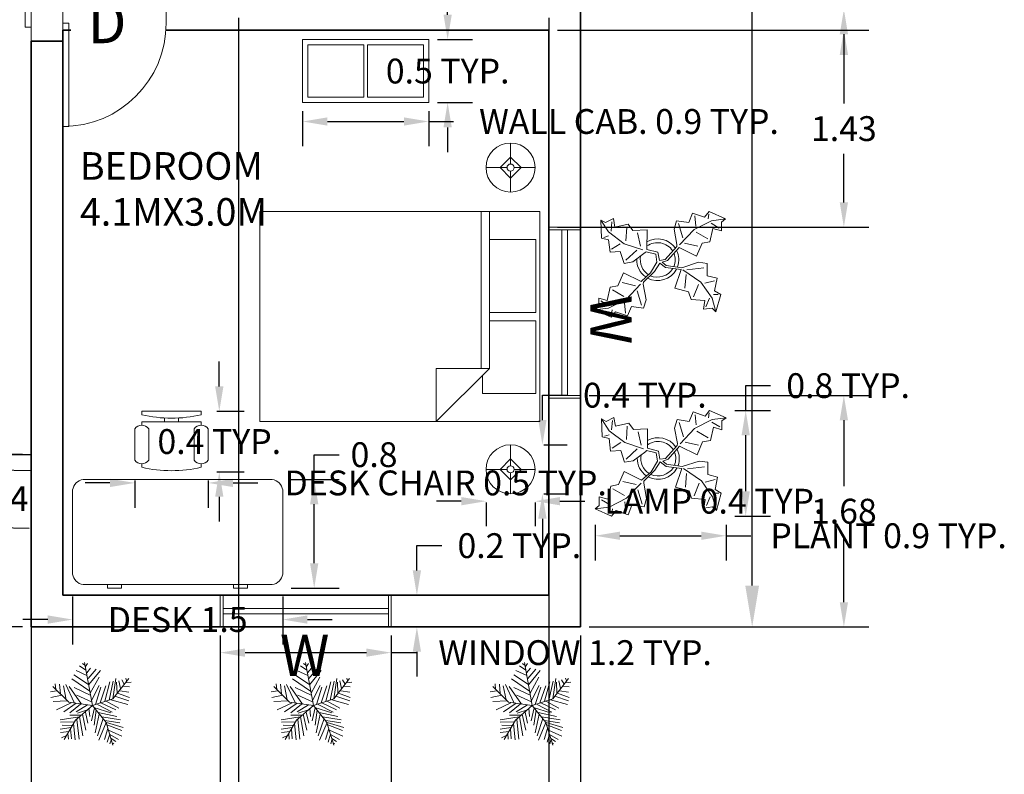
# Model space of a CAD drawing. Units: metres. Extents: x 40.9 to 56.1, y -1.4 to 24.2.
# Tile 4 of 7: x 48.4 to 55.6, y 7.6 to 13.1. Entities that reach past the tile are written whole.
import ezdxf

# ---------------------------------------------------------------- set-up
doc = ezdxf.new("R2010")
doc.units = ezdxf.units.M
doc.header["$MEASUREMENT"] = 0
for name, color, linetype, lineweight in [('A-ANNO-DIMS', 2, 'Continuous', 18), ('A-ANNO-TEXT', 7, 'Continuous', 18), ('A-AREA-IDEN', 7, 'Continuous', 18), ('A-DOOR', 3, 'Continuous', 18), ('A-FLOR', 7, 'Continuous', 25), ('A-FLOR-CASE', 9, 'Continuous', 18), ('A-FURN', 8, 'Continuous', 18), ('A-GLAZ', 4, 'Continuous', 18), ('A-WALL', 7, 'Continuous', 35), ('L-PLNT', 94, 'Continuous', 13)]:
    doc.layers.add(name, color=color, linetype=linetype, lineweight=lineweight)
doc.styles.get("Standard").update_dxf_attribs({"font": 'arial.ttf'})
doc.dimstyles.get("Standard").update_dxf_attribs({"dimtxt": 0.18, "dimasz": 0.18, "dimexe": 0.18, "dimexo": 0.0625, "dimgap": 0.09, "dimtad": 0, "dimtih": 1, "dimtoh": 1, "dimdec": 1, "dimzin": 0, "dimdsep": 46, "dimtxsty": 'Standard', "dimcen": 0.09, "dimadec": 0, "dimazin": 0, "dimtfac": 1, "dimtdec": 1, "dimtofl": 0, "dimtmove": 0, "dimatfit": 3, "dimfxl": 1, "dimtolj": 1, "dimtzin": 0, "dimarcsym": 0})

# ---------------------------------------------------------------- blocks, each defined once
blk = doc.blocks.new('*U3')
for p, q in [((-750, 0), (-750, -100)), ((0, 0), (0, -100))]:
    blk.add_line(p, q)
blk.add_lwpolyline([(0, 0), (0, 750), (-43.75, 750), (-43.75, 0)], close=True)
blk.add_arc((0, 0), 750, 90, 180)
blk = doc.blocks.new('*U4')
for p, q in [((0, 0), (0, 100)), ((750, 0), (750, 100))]:
    blk.add_line(p, q)
blk.add_lwpolyline([(0, 0), (0, -750), (43.75, -750), (43.75, 0)], close=True)
blk.add_arc((0, 0), 750, 270, 0)
blk = doc.blocks.new('Bed - Queen')
for p, q in [((0, -80.00003), (0, 0)), ((0, 0), (59.99999, 0)), ((59.99999, 0), (59.99999, -80.00003)), ((7.99999, -1.2), (28.79998, -1.2)), ((7.99999, -14.4), (7.99999, -1.2)), ((28.79998, -1.2), (28.79998, -14.4)), ((31.19999, -1.2), (51.99999, -1.2)), ((31.19999, -14.4), (31.19999, -1.2)), ((51.99999, -1.2), (51.99999, -16.4)), ((0, -14.4), (44.8, -14.4)), ((44.8, -16.8), (0, -16.8)), ((59.99999, -29.6), (44.8, -14.4)), ((44.8, -14.4), (44.8, -29.6)), ((51.99999, -16.4), (46.79936, -16.4)), ((44.8, -29.6), (59.99999, -29.6)), ((59.99999, -80.00003), (0, -80.00003))]:
    blk.add_line(p, q)
blk = doc.blocks.new('Lamp - Table')
for p, q in [((0, 7), (0, 1)), ((0, 3), (-3, 0)), ((3, 0), (0, 3)), ((-1, 0), (-7, 0)), ((-3, 0), (0, -3)), ((0, -3), (3, 0)), ((1, 0), (7, 0)), ((0, -1), (0, -7))]:
    blk.add_line(p, q)
for radius in [7, 1]:
    blk.add_circle((0, 0), radius)
blk = doc.blocks.new('Chair - Desk')
for p, q in [((-8.5, 0), (-8.5, -1)), ((-8.5, 0), (8.5, 0)), ((8.5, 0), (8.5, -1)), ((-2, -3), (-2, -1.9355)), ((2, -1.9576), (2, -3)), ((-10.5, -5), (-10.5, -14)), ((-8.5, -3), (-8.5, -4)), ((-8.5, -3), (8.5, -3)), ((-6.5, -14), (-6.5, -5)), ((6.5, -5), (6.5, -14)), ((8.5, -3), (8.5, -4)), ((10.5, -14), (10.5, -5)), ((-8.5, -15), (-8.5, -16)), ((8.5, -15), (8.5, -16))]:
    blk.add_line(p, q)
for centre, radius, start, end in [((0, 34.625), 36.625, 256.5803, 283.4197), ((-8.5, -6.5), 2.5, 36.8699, 143.1301), ((8.5, -6.5), 2.5, 36.8699, 143.1301), ((-8.5, -12.5), 2.5, 216.8699, 323.1301), ((8.5, -12.5), 2.5, 216.8699, 323.1301), ((0, 19.625), 36.625, 256.5803, 283.4197)]:
    blk.add_arc(centre, radius, start, end)
blk = doc.blocks.new('Desk - 30 x 60 in.')
for p, q in [((-26.999995, 0), (26.999995, 0)), ((-29.999995, -27), (-29.999995, -3)), ((29.999995, -3), (29.999995, -27)), ((26.999995, -30), (-26.999995, -30)), ((-20.000005, -30), (-20.000005, -31)), ((-16.000005, -31), (-16.000005, -30)), ((15.999995, -31), (15.999995, -30)), ((19.999995, -30), (19.999995, -31)), ((-20.000005, -31), (-16.000005, -31)), ((19.999995, -31), (15.999995, -31))]:
    blk.add_line(p, q)
for centre, start, end in [((-26.499995, -3.5), 98.1301, 171.8699), ((26.499995, -3.5), 8.130102, 81.8699), ((-26.499995, -26.5), 188.1301, 261.8699), ((26.499995, -26.5), 278.1301, 351.8699)]:
    blk.add_arc(centre, 3.535534, start, end)
blk = doc.blocks.new('Wall Cabinet - 18 x 36 in front')
for p, q in [((17.5, -1.5), (17.5, -16.5)), ((18.5, -16.5), (18.5, -1.5))]:
    blk.add_line(p, q)
blk.add_lwpolyline([(0, -18), (0, 0), (36, 0), (36, -18)], close=True)
for points in [[(17.5, -16.5), (1.5, -16.5), (1.5, -1.5), (17.5, -1.5)], [(18.5, -1.5), (34.5, -1.5), (34.5, -16.5), (18.5, -16.5)]]:
    blk.add_lwpolyline(points)
blk = doc.blocks.new('*U26')
for p, q in [((-221.9198, 1197.3052), (-433.5526, 1338.8594)), ((-258.7244, 1362.456), (-332.3336, 1421.4348)), ((0, 0), (-266.7, 1447.8)), ((-231.1146, 1315.2628), (-166.7002, 1421.4348)), ((-129.8956, 713.6638), (-626.7704, 1032.1544)), ((-185.1152, 1008.5578), (-553.1612, 1185.4942)), ((-194.31, 1102.9442), (-65.4812, 1256.284)), ((-148.3106, 914.1968), (118.5418, 1220.9018)), ((-129.8956, 701.8528), (265.7602, 1185.4942)), ((-1234.059, 536.7274), (-1252.4486, 737.2604)), ((-1105.2302, 725.4494), (-1077.6458, 395.1732)), ((-976.4268, 666.4706), (-884.4026, 194.6402)), ((-902.8176, 713.6638), (-617.5756, 100.2538)), ((-93.091, 489.5342), (-700.3796, 902.3858)), ((-74.7014, 418.7444), (219.7608, 961.39)), ((-28.6766, 171.0436), (228.9556, 678.2816)), ((256.5654, 88.4682), (449.7832, 666.4706)), ((412.9786, 147.447), (587.8068, 796.2392)), ((560.197, 182.8292), (698.2206, 819.8358)), ((685.8, 228.6), (1219.2, 914.4)), ((689.0258, 230.0224), (790.2448, 914.1968)), ((808.6344, 784.4282), (827.0494, 418.7444)), ((891.4384, 831.6214), (946.658, 572.1096)), ((983.4626, 867.0036), (1066.2666, 725.4494)), ((1112.2914, 760.8316), (1296.3144, 784.4282)), ((1121.4862, 925.9824), (1149.0706, 831.6214)), ((-1206.4492, 501.3198), (-1418.082, 465.9376)), ((-1031.621, 347.98), (-1399.667, 277.1902)), ((-800.1, 114.3), (-1333.5, 647.7)), ((-369.1382, 53.086), (-783.1836, 642.874)), ((-617.5756, 607.4918), (-74.7014, 347.98)), ((-525.5514, 347.98), (-28.6766, 123.8504)), ((100.1268, 41.275), (284.1498, 619.2774)), ((845.439, 418.7444), (1241.0948, 277.1902)), ((919.0482, 501.3198), (1222.6798, 454.152)), ((1029.462, 654.685), (1241.0948, 631.0884)), ((-847.598, 159.2326), (-1326.0578, 135.636)), ((-718.7946, 88.4682), (-1215.644, -147.447)), ((-543.9664, 76.6572), (-967.2066, -206.4512)), ((0, 0), (-800.1, 114.3)), ((-405.9428, 53.086), (-764.794, -241.8334)), ((0, 0), (-571.5, -495.3)), ((-166.7002, 29.4894), (-543.9664, -206.4512)), ((0, 0), (685.8, 228.6)), ((0, 0), (457.2, -571.5)), ((164.5412, 41.275), (661.416, -218.2368)), ((284.1498, 88.4682), (781.0246, -147.447)), ((458.978, 147.447), (891.4384, -88.4682)), ((615.4166, 194.6402), (1185.8752, 41.275)), ((753.4148, 312.5978), (1222.6798, 159.2326)), ((-387.5278, -324.4088), (-764.794, -324.4088)), ((-166.7002, -147.447), (-507.1618, -253.619)), ((-341.5284, -289.0012), (-221.9198, -831.6214)), ((-240.3094, -218.2368), (-157.5054, -595.7062)), ((-120.7008, -88.4682), (-93.091, -371.5766)), ((63.3222, -76.6826), (-37.8714, -513.1308)), ((44.9326, -64.897), (615.4166, -241.8334)), ((127.7366, -159.258), (54.1274, -654.685)), ((228.9556, -289.0012), (90.932, -914.1968)), ((192.151, -230.0224), (817.8292, -371.5766)), ((-442.7474, -383.3876), (-1086.8406, -477.7486)), ((-617.5756, -548.5384), (-1077.6458, -560.324)), ((-681.9646, -666.496), (-1022.4262, -654.685)), ((-571.5, -495.3), (-952.5, -1143)), ((-635.9652, -607.5172), (-580.771, -1150.1374)), ((-525.5514, -465.963), (-451.9422, -1126.5408)), ((-433.5526, -383.3876), (-323.1134, -1020.3688)), ((357.759, -430.5554), (164.5412, -1020.3688)), ((458.978, -572.1096), (210.5406, -1161.923)), ((311.7596, -383.3876), (937.4378, -477.7486)), ((412.9786, -501.3452), (919.0482, -583.9206)), ((457.2, -571.5), (685.8, -1333.5)), ((468.1982, -572.1096), (1029.462, -737.2604)), ((486.5878, -642.8994), (983.4626, -843.4324)), ((-718.7946, -737.2604), (-1086.8406, -796.2392)), ((-783.1836, -867.029), (-1077.6458, -902.4112)), ((-829.2084, -937.7934), (-810.7934, -1126.5408)), ((-737.1842, -784.4536), (-709.5744, -1114.7298)), ((514.1976, -772.6426), (403.7838, -1138.3264)), ((578.612, -961.39), (495.7826, -1232.7128)), ((541.8074, -831.6214), (992.6574, -1032.1544)), ((578.612, -973.1756), (873.0488, -1138.3264)), ((-875.2078, -1008.5832), (-1040.8412, -1079.3476)), ((624.6114, -1161.923), (587.8068, -1291.6916)), ((624.6114, -1102.9442), (781.0246, -1209.1162)), ((679.8056, -1268.095), (716.6102, -1291.6916))]:
    blk.add_line(p, q)
blk = doc.blocks.new('Plant - Rubber or Philodendron')
for p, q in [((-16.2005, 11.4774), (-13.9899, 8.1064)), ((-16.2005, 11.4774), (-14.8639, 10.7964)), ((-16.0159, 6.3329), (-16.2005, 11.4774)), ((-14.8639, 10.7964), (-12.6195, 11.8975)), ((-12.6195, 11.8975), (-12.1909, 9.4345)), ((4.6914, 8.8812), (5.3859, 11.2828)), ((5.3859, 11.2828), (8.8871, 10.7908)), ((8.8871, 10.7908), (9.9809, 13.4933)), ((9.9809, 13.4933), (13.3837, 12.301)), ((15.3859, 11.3055), (10.3916, 8.7942)), ((10.5828, 12.6946), (10.8893, 9.7953)), ((13.3837, 12.301), (14.68, 13.9039)), ((14.5816, 13.2037), (14.3848, 11.8033)), ((14.68, 13.9039), (19.3848, 11.8146)), ((19.3848, 11.8146), (15.3859, 11.3055)), ((19.3848, 11.8146), (18.1868, 10.9119)), ((-13.3174, 8.325), (-13.0735, 11.0065)), ((-12.1909, 9.4345), (-8.3829, 10.3)), ((-8.8369, 9.409), (-9.0894, 5.6095)), ((-8.3829, 10.3), (-7.0549, 8.501)), ((-7.0549, 8.501), (-3.0284, 8.6941)), ((-3.0284, 8.6941), (-3.0709, 3.1041)), ((4.6914, 8.8812), (5.5014, 4.4831)), ((5.9878, 10.4842), (7.1971, 6.3869)), ((10.3916, 8.7942), (6.2847, 4.4028)), ((15.7909, 9.1065), (14.8995, 5.3044)), ((15.2875, 10.6053), (17.5907, 9.2105)), ((18.1925, 8.4119), (15.7909, 9.1065)), ((18.1868, 10.9119), (18.1925, 8.4119)), ((-14.0069, 5.8704), (-16.0159, 6.3329)), ((-15.3434, 6.5514), (-13.9984, 6.9884)), ((-13.5868, 2.2894), (-14.0069, 5.8704)), ((-13.9899, 8.1064), (-9.5434, 4.7185)), ((-4.8529, 4.012), (-5.7184, 7.82)), ((14.2977, 6.1031), (10.9934, 7.9956)), ((-13.1329, 3.1804), (-10.6614, 4.727)), ((-9.5434, 4.7185), (-4.1917, 2.9888)), ((-9.1318, 0.0195), (-5.9793, 2.9025)), ((-3.0709, 3.1041), (0.0797, 2.3163)), ((2.1141, 0.2298), (5.4346, 3.9146)), ((6.1032, 3.6844), (2.8262, -0.031)), ((5.4346, 3.9146), (5.5014, 4.4831)), ((11.1089, 1.1958), (6.1032, 3.6844)), ((7.7005, 4.8881), (11.5025, 3.9967)), ((12.7005, 4.8994), (11.1089, 1.1958)), ((14.8995, 5.3044), (12.7005, 4.8994)), ((-10.6784, 2.491), (-13.5868, 2.2894)), ((-9.5858, -0.8715), (-10.6784, 2.491)), ((-7.1228, -0.443), (-3.5248, 2.2131)), ((-3.5248, 2.2131), (-3.3011, 2.4355)), ((-3.3011, 2.4355), (-0.5306, 1.7947)), ((-0.5306, 1.7947), (-0.2255, -0.5527)), ((-0.5306, 1.7947), (-0.5306, 1.7947)), ((0.0797, 2.3163), (0.4866, -0.031)), ((0.4866, -0.031), (2.1141, 0.2298)), ((-7.1228, -0.443), (-9.5858, -0.8715)), ((-2.019, -3.6148), (-0.2255, -0.5527)), ((-0.9375, -3.1608), (0.5883, -0.8135)), ((0.5883, -0.8135), (2.2447, -2.0916)), ((2.8262, -0.031), (1.3003, -0.5527)), ((1.3003, -0.5527), (2.4193, -1.4655)), ((2.2447, -2.0916), (6.7108, -2.6626)), ((2.4193, -1.4655), (6.895, -2.1175)), ((4.943, -7.9659), (6.7108, -2.6626)), ((11.6605, -0.5413), (6.895, -2.1175)), ((12.3677, -6.1981), (7.219, -2.6772)), ((8.3544, -2.7453), (13.1973, -2.1704)), ((11.6605, -0.5413), (14.1354, -0.8948)), ((14.1354, -0.8948), (14.1354, -4.4304)), ((-11.3237, -7.2629), (-9.7321, -3.5593)), ((-9.7321, -3.5593), (-4.7264, -6.0479)), ((-2.019, -3.6148), (-4.7264, -6.0479)), ((-4.0579, -6.2781), (-0.9375, -3.1608)), ((8.125, -4.0768), (7.7715, -7.9659)), ((14.1354, -4.4304), (16.9638, -5.1375)), ((16.9638, -5.1375), (16.2567, -8.673)), ((-14.4141, -11.4699), (-13.5228, -7.6679)), ((-13.5228, -7.6679), (-11.3237, -7.2629)), ((-6.3237, -7.2516), (-10.1257, -6.3602)), ((-9.0148, -11.1577), (-4.9047, -6.8122)), ((-4.1246, -6.8466), (-4.0579, -6.2781)), ((-3.3146, -11.2447), (-4.1246, -6.8466)), ((8.8321, -9.0266), (4.943, -7.9659)), ((10.2463, -10.4408), (11.6605, -6.9053)), ((15.5496, -10.7943), (12.3677, -6.1981)), ((16.2567, -5.8446), (13.4283, -6.5517)), ((-16.8157, -10.7754), (-14.4141, -11.4699)), ((-16.8101, -13.2754), (-16.8157, -10.7754)), ((-14.0091, -13.669), (-9.0148, -11.1577)), ((-12.921, -8.4665), (-9.6166, -10.359)), ((-4.611, -12.8477), (-5.8203, -8.7504)), ((-3.3146, -11.2447), (-4.0092, -13.6463)), ((9.5392, -11.1479), (8.8321, -9.0266)), ((13.4283, -11.5015), (9.5392, -11.1479)), ((14.8425, -10.7943), (13.7819, -13.2692)), ((16.6103, -14.6834), (15.5496, -10.7943)), ((17.3174, -9.7337), (15.9032, -9.7337)), ((16.2567, -8.673), (18.0245, -9.7337)), ((18.0245, -9.7337), (16.6103, -14.6834)), ((-18.008, -14.1781), (-16.8101, -13.2754)), ((-18.008, -14.1781), (-14.0091, -13.669)), ((-13.9107, -12.9688), (-16.2139, -11.574)), ((-9.206, -15.0581), (-9.5126, -12.1588)), ((-7.5103, -13.1543), (-8.6042, -15.8568)), ((-4.0092, -13.6463), (-7.5103, -13.1543)), ((13.0748, -13.9763), (13.4283, -11.5015)), ((15.5496, -13.6228), (13.0748, -13.9763)), ((16.6103, -14.6834), (15.5496, -13.6228)), ((-13.3032, -16.2674), (-18.008, -14.1781)), ((-12.0069, -14.6645), (-13.3032, -16.2674)), ((-13.2048, -15.5672), (-13.008, -14.1668)), ((-8.6042, -15.8568), (-12.0069, -14.6645))]:
    blk.add_line(p, q)
for centre, radius, start, end in [((0, 0), 6.1275, 34.37569, 120.1028), ((-0.0601, -0.2075), 5.2461, 33.82192, 124.9414), ((-0.098, 0.1364), 6.1288, 341.2017, 26.09184), ((0.0308, 0.1664), 6, 178.6147, 235.1169), ((0.0308, 0.1664), 5, 168.1647, 238.6725), ((-0.2664, 0.1682), 5.2775, 338.4094, 20.03007), ((-0.0234, 0.3825), 6.1492, 242.5812, 331.2714), ((-0.1102, 0.4886), 5.2883, 247.3711, 327.472)]:
    blk.add_arc(centre, radius, start, end)
blk = doc.blocks.new('*D46')
at = {"layer": 'A-ANNO-DIMS', "color": 0, "lineweight": -2, "transparency": 16777216}
for p, q in [((52.5777, 22.5873), (53.9408, 22.5873)), ((53.7608, 22.2873), (53.7608, 15.8755)), ((53.7608, 8.9773), (53.7608, 15.389)), ((52.5777, 8.6773), (53.9408, 8.6773))]:
    blk.add_line(p, q, dxfattribs=at)
at = {"layer": 'A-ANNO-DIMS', "color": 0, "transparency": 16777216}
for points in [[(53.7108, 22.2873), (53.8108, 22.2873), (53.7608, 22.5873)], [(53.7108, 8.9773), (53.8108, 8.9773), (53.7608, 8.6773)]]:
    blk.add_solid(points, dxfattribs=at)
at = {"layer": 'Defpoints', "color": 0, "transparency": 16777216}
for p in [(52.5152, 22.5873), (52.5152, 8.6773), (53.7608, 8.6773)]:
    blk.add_point(p, dxfattribs=at)
at = {"layer": 'A-ANNO-DIMS', "color": 0, "transparency": 16777216, "insert": (53.7608, 15.6323), "char_height": 0.3, "attachment_point": 5}
blk.add_mtext('\\A1;13.9', dxfattribs=at)
blk = doc.blocks.new('WIN-1200-PLAN')
for p, q in [((-0.0002, 0.0003), (-0.0002, 0.2303)), ((0.0198, 0.0003), (0.0198, 0.2303)), ((1.2198, 0.0003), (1.2198, 0.2303)), ((1.2398, 0.0003), (1.2398, 0.2303)), ((0.0198, 0.1353), (1.2198, 0.1353)), ((0.0198, 0.0953), (1.2198, 0.0953))]:
    blk.add_line(p, q)
blk = doc.blocks.new('*D73')
at = {"layer": 'A-ANNO-DIMS', "color": 0, "lineweight": -2, "transparency": 16777216}
for p, q in [((49.9027, 8.6148), (49.9027, 8.3113)), ((51.1427, 8.6148), (51.1427, 8.3113)), ((50.0827, 8.4913), (50.9627, 8.4913)), ((51.1427, 8.4913), (51.3227, 8.4913))]:
    blk.add_line(p, q, dxfattribs=at)
at = {"layer": 'A-ANNO-DIMS', "color": 0, "transparency": 16777216}
for points in [[(50.0827, 8.5213), (50.0827, 8.4613), (49.9027, 8.4913)], [(50.9627, 8.5213), (50.9627, 8.4613), (51.1427, 8.4913)]]:
    blk.add_solid(points, dxfattribs=at)
at = {"layer": 'Defpoints', "color": 0, "transparency": 16777216}
for p in [(49.9027, 8.6773), (51.1427, 8.6773), (51.1427, 8.4913)]:
    blk.add_point(p, dxfattribs=at)
at = {"layer": 'A-ANNO-DIMS', "color": 0, "transparency": 16777216, "insert": (52.476, 8.4913), "char_height": 0.18, "attachment_point": 5}
blk.add_mtext('\\A1;WINDOW 1.2 TYP.', dxfattribs=at)
blk = doc.blocks.new('*D74')
at = {"layer": 'A-ANNO-DIMS', "color": 0, "lineweight": -2, "transparency": 16777216}
for p, q in [((51.3287, 9.0873), (51.3287, 9.2673)), ((51.3287, 9.2673), (51.5087, 9.2673)), ((51.2052, 8.9073), (51.5087, 8.9073)), ((51.2052, 8.6773), (51.5087, 8.6773)), ((51.3287, 8.4973), (51.3287, 8.3173))]:
    blk.add_line(p, q, dxfattribs=at)
at = {"layer": 'A-ANNO-DIMS', "color": 0, "transparency": 16777216}
for points in [[(51.2987, 9.0873), (51.3587, 9.0873), (51.3287, 8.9073)], [(51.2987, 8.4973), (51.3587, 8.4973), (51.3287, 8.6773)]]:
    blk.add_solid(points, dxfattribs=at)
at = {"layer": 'Defpoints', "color": 0, "transparency": 16777216}
for p in [(51.1427, 8.9073), (51.3287, 8.9073), (51.1427, 8.6773)]:
    blk.add_point(p, dxfattribs=at)
at = {"layer": 'A-ANNO-DIMS', "color": 0, "transparency": 16777216, "insert": (52.0717, 9.2673), "char_height": 0.18, "attachment_point": 5}
blk.add_mtext('\\A1;0.2 TYP.', dxfattribs=at)
blk = doc.blocks.new('*D81')
at = {"layer": 'A-ANNO-DIMS', "color": 0, "lineweight": -2, "transparency": 16777216}
for p, q in [((51.6504, 9.5897), (51.4704, 9.5897)), ((51.8304, 9.5805), (51.8304, 9.4097)), ((52.186, 9.5805), (52.186, 9.4097)), ((52.366, 9.5897), (52.546, 9.5897))]:
    blk.add_line(p, q, dxfattribs=at)
at = {"layer": 'A-ANNO-DIMS', "color": 0, "transparency": 16777216}
for points in [[(51.6504, 9.6197), (51.6504, 9.5597), (51.8304, 9.5897)], [(52.366, 9.6197), (52.366, 9.5597), (52.186, 9.5897)]]:
    blk.add_solid(points, dxfattribs=at)
at = {"layer": 'Defpoints', "color": 0, "transparency": 16777216}
for p in [(51.8304, 9.643), (52.186, 9.643), (52.186, 9.5897)]:
    blk.add_point(p, dxfattribs=at)
at = {"layer": 'A-ANNO-DIMS', "color": 0, "transparency": 16777216, "insert": (53.4823, 9.5897), "char_height": 0.18, "attachment_point": 5}
blk.add_mtext('\\A1;LAMP 0.4 TYP.', dxfattribs=at)
blk = doc.blocks.new('*D82')
at = {"layer": 'A-ANNO-DIMS', "color": 0, "lineweight": -2, "transparency": 16777216}
for p, q in [((52.2393, 10.1786), (52.2393, 10.3586)), ((52.2393, 10.3586), (52.4193, 10.3586)), ((52.2485, 9.9986), (52.4193, 9.9986)), ((52.2485, 9.643), (52.4193, 9.643)), ((52.2393, 9.463), (52.2393, 9.283))]:
    blk.add_line(p, q, dxfattribs=at)
at = {"layer": 'A-ANNO-DIMS', "color": 0, "transparency": 16777216}
for points in [[(52.2093, 10.1786), (52.2693, 10.1786), (52.2393, 9.9986)], [(52.2093, 9.463), (52.2693, 9.463), (52.2393, 9.643)]]:
    blk.add_solid(points, dxfattribs=at)
at = {"layer": 'Defpoints', "color": 0, "transparency": 16777216}
for p in [(52.186, 9.9986), (52.2393, 9.9986), (52.186, 9.643)]:
    blk.add_point(p, dxfattribs=at)
at = {"layer": 'A-ANNO-DIMS', "color": 0, "transparency": 16777216, "insert": (52.9824, 10.3586), "char_height": 0.18, "attachment_point": 5}
blk.add_mtext('\\A1;0.4 TYP.', dxfattribs=at)
blk = doc.blocks.new('*D83')
at = {"layer": 'A-ANNO-DIMS', "color": 0, "lineweight": -2, "transparency": 16777216}
for p, q in [((49.1021, 9.7223), (48.9221, 9.7223)), ((49.2821, 9.7398), (49.2821, 9.5423)), ((49.8155, 9.7398), (49.8155, 9.5423)), ((49.9955, 9.7223), (50.1755, 9.7223))]:
    blk.add_line(p, q, dxfattribs=at)
at = {"layer": 'A-ANNO-DIMS', "color": 0, "transparency": 16777216}
for points in [[(49.1021, 9.7523), (49.1021, 9.6923), (49.2821, 9.7223)], [(49.9955, 9.7523), (49.9955, 9.6923), (49.8155, 9.7223)]]:
    blk.add_solid(points, dxfattribs=at)
at = {"layer": 'Defpoints', "color": 0, "transparency": 16777216}
for p in [(49.2821, 9.8023), (49.8155, 9.8023), (49.8155, 9.7223)]:
    blk.add_point(p, dxfattribs=at)
at = {"layer": 'A-ANNO-DIMS', "color": 0, "transparency": 16777216, "insert": (51.5375, 9.7223), "char_height": 0.18, "attachment_point": 5}
blk.add_mtext('\\A1;DESK CHAIR 0.5 TYP.', dxfattribs=at)
blk = doc.blocks.new('*D84')
at = {"layer": 'A-ANNO-DIMS', "color": 0, "lineweight": -2, "transparency": 16777216}
for p, q in [((49.8955, 10.4226), (49.8955, 10.6026)), ((49.878, 10.2426), (50.0755, 10.2426)), ((49.878, 9.8023), (50.0755, 9.8023)), ((49.8955, 9.6223), (49.8955, 9.4423))]:
    blk.add_line(p, q, dxfattribs=at)
at = {"layer": 'A-ANNO-DIMS', "color": 0, "transparency": 16777216}
for points in [[(49.8655, 10.4226), (49.9255, 10.4226), (49.8955, 10.2426)], [(49.8655, 9.6223), (49.9255, 9.6223), (49.8955, 9.8023)]]:
    blk.add_solid(points, dxfattribs=at)
at = {"layer": 'Defpoints', "color": 0, "transparency": 16777216}
for p in [(49.8155, 10.2426), (49.8955, 10.2426), (49.8155, 9.8023)]:
    blk.add_point(p, dxfattribs=at)
at = {"layer": 'A-ANNO-DIMS', "color": 0, "transparency": 16777216, "insert": (49.8955, 10.0225), "char_height": 0.18, "attachment_point": 5}
blk.add_mtext('\\A1;0.4 TYP.', dxfattribs=at)
blk = doc.blocks.new('*D85')
at = {"layer": 'A-ANNO-DIMS', "color": 0, "lineweight": -2, "transparency": 16777216}
for p, q in [((50.5003, 12.4186), (50.5003, 12.1639)), ((51.4147, 12.4186), (51.4147, 12.1639)), ((50.6803, 12.3439), (51.2347, 12.3439)), ((51.4147, 12.3439), (51.5947, 12.3439))]:
    blk.add_line(p, q, dxfattribs=at)
at = {"layer": 'A-ANNO-DIMS', "color": 0, "transparency": 16777216}
for points in [[(50.6803, 12.3739), (50.6803, 12.3139), (50.5003, 12.3439)], [(51.2347, 12.3739), (51.2347, 12.3139), (51.4147, 12.3439)]]:
    blk.add_solid(points, dxfattribs=at)
at = {"layer": 'Defpoints', "color": 0, "transparency": 16777216}
for p in [(50.5003, 12.4811), (51.4147, 12.4811), (51.4147, 12.3439)]:
    blk.add_point(p, dxfattribs=at)
at = {"layer": 'A-ANNO-DIMS', "color": 0, "transparency": 16777216, "insert": (52.8671, 12.3439), "char_height": 0.18, "attachment_point": 5}
blk.add_mtext('\\A1;WALL CAB. 0.9 TYP.', dxfattribs=at)
blk = doc.blocks.new('*D86')
at = {"layer": 'A-ANNO-DIMS', "color": 0, "lineweight": -2, "transparency": 16777216}
for p, q in [((51.5519, 13.1183), (51.5519, 13.2983)), ((51.4772, 12.9383), (51.7319, 12.9383)), ((51.4772, 12.4811), (51.7319, 12.4811)), ((51.5519, 12.3011), (51.5519, 12.1211))]:
    blk.add_line(p, q, dxfattribs=at)
at = {"layer": 'A-ANNO-DIMS', "color": 0, "transparency": 16777216}
for points in [[(51.5219, 13.1183), (51.5819, 13.1183), (51.5519, 12.9383)], [(51.5219, 12.3011), (51.5819, 12.3011), (51.5519, 12.4811)]]:
    blk.add_solid(points, dxfattribs=at)
at = {"layer": 'Defpoints', "color": 0, "transparency": 16777216}
for p in [(51.4147, 12.9383), (51.5519, 12.9383), (51.4147, 12.4811)]:
    blk.add_point(p, dxfattribs=at)
at = {"layer": 'A-ANNO-DIMS', "color": 0, "transparency": 16777216, "insert": (51.5519, 12.7097), "char_height": 0.18, "attachment_point": 5}
blk.add_mtext('\\A1;0.5 TYP.', dxfattribs=at)
blk = doc.blocks.new('*D89')
at = {"layer": 'A-ANNO-DIMS', "color": 0, "lineweight": -2, "transparency": 16777216}
for p, q in [((52.6216, 9.419), (52.6216, 9.159)), ((53.5713, 9.419), (53.5713, 9.159)), ((52.8016, 9.339), (53.3913, 9.339)), ((53.5713, 9.339), (53.7513, 9.339))]:
    blk.add_line(p, q, dxfattribs=at)
at = {"layer": 'A-ANNO-DIMS', "color": 0, "transparency": 16777216}
for points in [[(52.8016, 9.369), (52.8016, 9.309), (52.6216, 9.339)], [(53.3913, 9.369), (53.3913, 9.309), (53.5713, 9.339)]]:
    blk.add_solid(points, dxfattribs=at)
at = {"layer": 'Defpoints', "color": 0, "transparency": 16777216}
for p in [(52.6216, 9.4815), (53.5713, 9.4815), (53.5713, 9.339)]:
    blk.add_point(p, dxfattribs=at)
at = {"layer": 'A-ANNO-DIMS', "color": 0, "transparency": 16777216, "insert": (54.7501, 9.339), "char_height": 0.18, "attachment_point": 5}
blk.add_mtext('\\A1;PLANT 0.9 TYP.', dxfattribs=at)
blk = doc.blocks.new('*D90')
at = {"layer": 'A-ANNO-DIMS', "color": 0, "lineweight": -2, "transparency": 16777216}
for p, q in [((53.7138, 10.2479), (53.7138, 10.4279)), ((53.7138, 10.4279), (53.8938, 10.4279)), ((53.6338, 10.2479), (53.8938, 10.2479)), ((53.7138, 9.6615), (53.7138, 10.0679)), ((53.6338, 9.4815), (53.8938, 9.4815))]:
    blk.add_line(p, q, dxfattribs=at)
at = {"layer": 'A-ANNO-DIMS', "color": 0, "transparency": 16777216}
for points in [[(53.6838, 10.0679), (53.7438, 10.0679), (53.7138, 10.2479)], [(53.6838, 9.6615), (53.7438, 9.6615), (53.7138, 9.4815)]]:
    blk.add_solid(points, dxfattribs=at)
at = {"layer": 'Defpoints', "color": 0, "transparency": 16777216}
for p in [(53.5713, 10.2479), (53.7138, 10.2479), (53.5713, 9.4815)]:
    blk.add_point(p, dxfattribs=at)
at = {"layer": 'A-ANNO-DIMS', "color": 0, "transparency": 16777216, "insert": (54.4568, 10.4279), "char_height": 0.18, "attachment_point": 5}
blk.add_mtext('\\A1;0.8 TYP.', dxfattribs=at)
blk = doc.blocks.new('*D103')
at = {"layer": 'A-ANNO-DIMS', "color": 0, "lineweight": -2, "transparency": 16777216}
for p, q in [((48.8314, 8.8973), (48.8314, 8.5512)), ((50.3554, 8.8973), (50.3554, 8.5512)), ((48.6514, 8.7312), (48.4714, 8.7312)), ((50.5354, 8.7312), (50.7154, 8.7312))]:
    blk.add_line(p, q, dxfattribs=at)
at = {"layer": 'A-ANNO-DIMS', "color": 0, "transparency": 16777216}
for points in [[(48.6514, 8.7612), (48.6514, 8.7012), (48.8314, 8.7312)], [(50.5354, 8.7612), (50.5354, 8.7012), (50.3554, 8.7312)]]:
    blk.add_solid(points, dxfattribs=at)
at = {"layer": 'Defpoints', "color": 0, "transparency": 16777216}
for p in [(48.8314, 8.9598), (50.3554, 8.9598), (50.3554, 8.7312)]:
    blk.add_point(p, dxfattribs=at)
at = {"layer": 'A-ANNO-DIMS', "color": 0, "transparency": 16777216, "insert": (49.5934, 8.7312), "char_height": 0.18, "attachment_point": 5}
blk.add_mtext('\\A1;DESK 1.5', dxfattribs=at)
blk = doc.blocks.new('*D104')
at = {"layer": 'A-ANNO-DIMS', "color": 0, "lineweight": -2, "transparency": 16777216}
for p, q in [((50.584, 9.7472), (50.584, 9.9272)), ((50.584, 9.9272), (50.764, 9.9272)), ((50.4179, 9.7472), (50.764, 9.7472)), ((50.584, 9.1398), (50.584, 9.5672)), ((50.4179, 8.9598), (50.764, 8.9598))]:
    blk.add_line(p, q, dxfattribs=at)
at = {"layer": 'A-ANNO-DIMS', "color": 0, "transparency": 16777216}
for points in [[(50.554, 9.5672), (50.614, 9.5672), (50.584, 9.7472)], [(50.554, 9.1398), (50.614, 9.1398), (50.584, 8.9598)]]:
    blk.add_solid(points, dxfattribs=at)
at = {"layer": 'Defpoints', "color": 0, "transparency": 16777216}
for p in [(50.3554, 9.7472), (50.584, 9.7472), (50.3554, 8.9598)]:
    blk.add_point(p, dxfattribs=at)
at = {"layer": 'A-ANNO-DIMS', "color": 0, "transparency": 16777216, "insert": (51.018, 9.9272), "char_height": 0.18, "attachment_point": 5}
blk.add_mtext('\\A1;0.8', dxfattribs=at)
blk = doc.blocks.new('*D114')
at = {"layer": 'A-ANNO-DIMS', "color": 0, "lineweight": -2, "transparency": 16777216}
for p, q in [((48.3498, 9.997), (48.3536, 10.177)), ((48.279, 9.8185), (48.526, 9.8133)), ((48.2702, 9.3995), (48.5172, 9.3943)), ((48.3335, 9.2181), (48.3297, 9.0381))]:
    blk.add_line(p, q, dxfattribs=at)
at = {"layer": 'A-ANNO-DIMS', "color": 0, "transparency": 16777216}
for points in [[(48.3198, 9.9977), (48.3798, 9.9964), (48.346, 9.8171)], [(48.3035, 9.2187), (48.3635, 9.2175), (48.3373, 9.3981)]]:
    blk.add_solid(points, dxfattribs=at)
at = {"layer": 'Defpoints', "color": 0, "transparency": 16777216}
for p in [(48.2165, 9.8198), (48.346, 9.8171), (48.2077, 9.4008)]:
    blk.add_point(p, dxfattribs=at)
at = {"layer": 'A-ANNO-DIMS', "color": 0, "transparency": 16777216, "insert": (48.3416, 9.6076), "char_height": 0.18, "attachment_point": 5}
blk.add_mtext('\\A1;0.4', dxfattribs=at)
blk = doc.blocks.new('*D129')
at = {"layer": 'A-ANNO-DIMS', "color": 0, "lineweight": -2, "transparency": 16777216}
for p, q in [((51.1427, 8.6148), (51.1427, 6.6791)), ((52.5152, 8.6148), (52.5152, 6.6791)), ((51.3227, 6.8591), (51.5136, 6.8591)), ((52.3352, 6.8591), (52.1443, 6.8591))]:
    blk.add_line(p, q, dxfattribs=at)
at = {"layer": 'A-ANNO-DIMS', "color": 0, "transparency": 16777216}
for points in [[(51.3227, 6.8891), (51.3227, 6.8291), (51.1427, 6.8591)], [(52.3352, 6.8891), (52.3352, 6.8291), (52.5152, 6.8591)]]:
    blk.add_solid(points, dxfattribs=at)
at = {"layer": 'Defpoints', "color": 0, "transparency": 16777216}
for p in [(51.1427, 8.6773), (52.5152, 8.6773), (52.5152, 6.8591)]:
    blk.add_point(p, dxfattribs=at)
at = {"layer": 'A-ANNO-DIMS', "color": 0, "transparency": 16777216, "insert": (51.829, 6.8591), "char_height": 0.18, "attachment_point": 5}
blk.add_mtext('\\A1;1.37', dxfattribs=at)
blk = doc.blocks.new('*D131')
at = {"layer": 'A-ANNO-DIMS', "color": 0, "lineweight": -2, "transparency": 16777216}
for p, q in [((48.4677, 9.9273), (43.1421, 9.9273)), ((43.3221, 9.7473), (43.3221, 9.4842)), ((43.3221, 8.8573), (43.3221, 9.1203)), ((48.4677, 8.6773), (43.1421, 8.6773))]:
    blk.add_line(p, q, dxfattribs=at)
at = {"layer": 'A-ANNO-DIMS', "color": 0, "transparency": 16777216}
for points in [[(43.2921, 9.7473), (43.3521, 9.7473), (43.3221, 9.9273)], [(43.2921, 8.8573), (43.3521, 8.8573), (43.3221, 8.6773)]]:
    blk.add_solid(points, dxfattribs=at)
at = {"layer": 'Defpoints', "color": 0, "transparency": 16777216}
for p in [(43.3221, 9.9273), (48.5302, 9.9273), (48.5302, 8.6773)]:
    blk.add_point(p, dxfattribs=at)
at = {"layer": 'A-ANNO-DIMS', "color": 0, "transparency": 16777216, "insert": (43.3221, 9.3023), "char_height": 0.18, "attachment_point": 5}
blk.add_mtext('\\A1;1.25', dxfattribs=at)
blk = doc.blocks.new('*D134')
at = {"layer": 'A-ANNO-DIMS', "color": 0, "lineweight": -2, "transparency": 16777216}
for p, q in [((50.034, 13.0948), (50.034, 6.6791)), ((52.2852, 13.0948), (52.2852, 6.6791)), ((50.214, 6.8591), (50.8336, 6.8591)), ((52.1052, 6.8591), (51.4856, 6.8591))]:
    blk.add_line(p, q, dxfattribs=at)
at = {"layer": 'A-ANNO-DIMS', "color": 0, "transparency": 16777216}
for points in [[(50.214, 6.8891), (50.214, 6.8291), (50.034, 6.8591)], [(52.1052, 6.8891), (52.1052, 6.8291), (52.2852, 6.8591)]]:
    blk.add_solid(points, dxfattribs=at)
at = {"layer": 'Defpoints', "color": 0, "transparency": 16777216}
for p in [(50.034, 13.1573), (52.2852, 13.1573), (52.2852, 6.8591)]:
    blk.add_point(p, dxfattribs=at)
at = {"layer": 'A-ANNO-DIMS', "color": 0, "transparency": 16777216, "insert": (51.1596, 6.8591), "char_height": 0.18, "attachment_point": 5}
blk.add_mtext('\\A1;2.25', dxfattribs=at)
blk = doc.blocks.new('*D139')
at = {"layer": 'A-ANNO-DIMS', "color": 0, "lineweight": -2, "transparency": 16777216}
for p, q in [((52.5777, 10.3573), (54.6058, 10.3573)), ((54.4258, 10.1773), (54.4258, 9.6992)), ((54.4258, 8.8573), (54.4258, 9.3353)), ((52.5777, 8.6773), (54.6058, 8.6773))]:
    blk.add_line(p, q, dxfattribs=at)
at = {"layer": 'A-ANNO-DIMS', "color": 0, "transparency": 16777216}
for points in [[(54.3958, 10.1773), (54.4558, 10.1773), (54.4258, 10.3573)], [(54.3958, 8.8573), (54.4558, 8.8573), (54.4258, 8.6773)]]:
    blk.add_solid(points, dxfattribs=at)
at = {"layer": 'Defpoints', "color": 0, "transparency": 16777216}
for p in [(52.5152, 10.3573), (54.4258, 10.3573), (52.5152, 8.6773)]:
    blk.add_point(p, dxfattribs=at)
at = {"layer": 'A-ANNO-DIMS', "color": 0, "transparency": 16777216, "insert": (54.4258, 9.5173), "char_height": 0.18, "attachment_point": 5}
blk.add_mtext('\\A1;1.68', dxfattribs=at)
blk = doc.blocks.new('*D148')
at = {"layer": 'A-ANNO-DIMS', "color": 0, "lineweight": -2, "transparency": 16777216}
for p, q in [((48.5302, 8.6148), (48.5302, 6.6791)), ((49.9027, 8.6148), (49.9027, 6.6791)), ((48.7102, 6.8591), (48.9011, 6.8591)), ((49.7227, 6.8591), (49.5318, 6.8591))]:
    blk.add_line(p, q, dxfattribs=at)
at = {"layer": 'A-ANNO-DIMS', "color": 0, "transparency": 16777216}
for points in [[(48.7102, 6.8891), (48.7102, 6.8291), (48.5302, 6.8591)], [(49.7227, 6.8891), (49.7227, 6.8291), (49.9027, 6.8591)]]:
    blk.add_solid(points, dxfattribs=at)
at = {"layer": 'Defpoints', "color": 0, "transparency": 16777216}
for p in [(48.5302, 8.6773), (49.9027, 8.6773), (49.9027, 6.8591)]:
    blk.add_point(p, dxfattribs=at)
at = {"layer": 'A-ANNO-DIMS', "color": 0, "transparency": 16777216, "insert": (49.2165, 6.8591), "char_height": 0.18, "attachment_point": 5}
blk.add_mtext('\\A1;1.37', dxfattribs=at)
blk = doc.blocks.new('*D152')
at = {"layer": 'A-ANNO-DIMS', "color": 0, "lineweight": -2, "transparency": 16777216}
for p, q in [((54.42584, 13.717253), (54.42584, 13.897253)), ((52.347703, 13.537253), (54.60584, 13.537253)), ((52.347703, 13.157253), (54.60584, 13.157253)), ((54.42584, 12.977253), (54.42584, 12.797253))]:
    blk.add_line(p, q, dxfattribs=at)
at = {"layer": 'A-ANNO-DIMS', "color": 0, "transparency": 16777216}
for points in [[(54.39584, 13.717253), (54.45584, 13.717253), (54.42584, 13.537253)], [(54.39584, 12.977253), (54.45584, 12.977253), (54.42584, 13.157253)]]:
    blk.add_solid(points, dxfattribs=at)
at = {"layer": 'Defpoints', "color": 0, "transparency": 16777216}
for p in [(52.285203, 13.537253), (54.42584, 13.537253), (52.285203, 13.157253)]:
    blk.add_point(p, dxfattribs=at)
at = {"layer": 'A-ANNO-DIMS', "color": 0, "transparency": 16777216, "insert": (54.42584, 13.347253), "char_height": 0.18, "attachment_point": 5}
blk.add_mtext('\\A1;0.38', dxfattribs=at)
blk = doc.blocks.new('*D156')
at = {"layer": 'A-ANNO-DIMS', "color": 0, "lineweight": -2, "transparency": 16777216}
for p, q in [((47.786899, 12.864753), (47.786899, 6.679084)), ((48.530203, 12.864753), (48.530203, 6.679084)), ((47.606899, 6.859084), (47.426899, 6.859084)), ((48.710203, 6.859084), (48.890203, 6.859084))]:
    blk.add_line(p, q, dxfattribs=at)
at = {"layer": 'A-ANNO-DIMS', "color": 0, "transparency": 16777216}
for points in [[(47.606899, 6.889084), (47.606899, 6.829084), (47.786899, 6.859084)], [(48.710203, 6.889084), (48.710203, 6.829084), (48.530203, 6.859084)]]:
    blk.add_solid(points, dxfattribs=at)
at = {"layer": 'Defpoints', "color": 0, "transparency": 16777216}
for p in [(47.786899, 12.927253), (48.530203, 12.927253), (48.530203, 6.859084)]:
    blk.add_point(p, dxfattribs=at)
at = {"layer": 'A-ANNO-DIMS', "color": 0, "transparency": 16777216, "insert": (48.158551, 6.859084), "char_height": 0.18, "attachment_point": 5}
blk.add_mtext('\\A1;0.74', dxfattribs=at)
blk = doc.blocks.new('*D160')
at = {"layer": 'A-ANNO-DIMS', "color": 0, "lineweight": -2, "transparency": 16777216}
for p, q in [((52.3477, 13.0073), (54.6058, 13.0073)), ((54.4258, 12.8273), (54.4258, 12.4742)), ((54.4258, 11.7573), (54.4258, 12.1103)), ((52.3477, 11.5773), (54.6058, 11.5773))]:
    blk.add_line(p, q, dxfattribs=at)
at = {"layer": 'A-ANNO-DIMS', "color": 0, "transparency": 16777216}
for points in [[(54.3958, 12.8273), (54.4558, 12.8273), (54.4258, 13.0073)], [(54.3958, 11.7573), (54.4558, 11.7573), (54.4258, 11.5773)]]:
    blk.add_solid(points, dxfattribs=at)
at = {"layer": 'Defpoints', "color": 0, "transparency": 16777216}
for p in [(52.2852, 13.0073), (54.4258, 13.0073), (52.2852, 11.5773)]:
    blk.add_point(p, dxfattribs=at)
at = {"layer": 'A-ANNO-DIMS', "color": 0, "transparency": 16777216, "insert": (54.4258, 12.2923), "char_height": 0.18, "attachment_point": 5}
blk.add_mtext('\\A1;1.43', dxfattribs=at)

msp = doc.modelspace()

# ---------------------------------------------------------------- linework, layer by layer
at = {"layer": 'A-FLOR'}
msp.add_line((45.2552, 9.9273), (48.5302, 9.9273), dxfattribs=at)
at = {"layer": 'A-WALL'}
for p, q in [((52.5152, 8.6773), (52.5152, 13.1573)), ((48.7602, 13.0073), (48.8179, 13.0073)), ((48.7602, 13.0073), (48.7602, 12.9273)), ((49.5085, 13.0073), (52.2852, 13.0073)), ((52.2852, 8.9073), (52.2852, 13.0073)), ((48.5302, 8.6773), (48.5302, 12.9273)), ((48.5302, 12.9273), (48.7602, 12.9273)), ((48.7602, 8.9073), (48.7602, 12.9273)), ((48.7602, 8.9073), (52.2852, 8.9073)), ((48.7602, 8.6773), (48.5302, 8.6773)), ((48.7602, 8.6773), (52.5152, 8.6773))]:
    msp.add_line(p, q, dxfattribs=at)

# ---------------------------------------------------------------- block references
at = {"layer": 'A-DOOR', "xscale": 0.001, "yscale": 0.001, "zscale": 0.001}
for name, p in [('*U3', (48.5302, 13.0273)), ('*U4', (48.7602, 13.0573))]:
    msp.add_blockref(name, p, dxfattribs=at)
at = {"layer": 'A-FLOR-CASE', "xscale": 0.0254, "yscale": 0.0254, "zscale": 0.0254}
msp.add_blockref('Wall Cabinet - 18 x 36 in front', (50.5003, 12.9383), dxfattribs=at)
at = {"layer": 'A-FURN', "xscale": 0.0254, "yscale": 0.0254, "zscale": 0.0254}
for name, p in [('Lamp - Table', (52.0082, 12.0099)), ('Chair - Desk', (49.5488, 10.2426)), ('Lamp - Table', (52.0082, 9.8208)), ('Desk - 30 x 60 in.', (49.5934, 9.7472))]:
    msp.add_blockref(name, p, dxfattribs=at)
at = {"layer": 'A-FURN', "xscale": 0.0254, "yscale": 0.0254, "zscale": 0.0254, "rotation": 270}
msp.add_blockref('Bed - Queen', (52.2217, 11.6908), dxfattribs=at)
at = {"layer": 'A-GLAZ', "rotation": 270.0000000000001}
msp.add_blockref('WIN-1200-PLAN', (52.2849, 11.5771), dxfattribs=at)
at = {"layer": 'A-GLAZ'}
msp.add_blockref('WIN-1200-PLAN', (49.9029, 8.677), dxfattribs=at)
at = {"layer": 'L-PLNT'}
for name, p, xscale, yscale, zscale in [('Plant - Rubber or Philodendron', (53.0751, 11.3369), 0.0254, 0.0254, 0.0254), ('Plant - Rubber or Philodendron', (53.079, 9.8947), 0.0254, 0.0254, 0.0254), ('*U26', (48.9759, 8.1071), 0.0002155130992256, 0.0002155130992256, 0.0002155130992256), ('*U26', (50.5782, 8.1071), 0.0002155130992256, 0.0002155130992256, 0.0002155130992256), ('*U26', (52.1661, 8.1071), 0.0002155130992256, 0.0002155130992256, 0.0002155130992256)]:
    msp.add_blockref(name, p, dxfattribs=dict(at, xscale=xscale, yscale=yscale, zscale=zscale))

# ---------------------------------------------------------------- texts
at = {"layer": 'A-ANNO-TEXT'}
for s, p in [('D ', (48.9405, 12.9118)), ('W', (50.3355, 8.3211))]:
    msp.add_text(s, height=0.3, dxfattribs=at).set_placement(p)
msp.add_text('W', height=0.3, rotation=270, dxfattribs=at).set_placement((52.5874, 11.0865))
at = {"layer": 'A-AREA-IDEN', "insert": (48.8846, 12.1214), "char_height": 0.2, "attachment_point": 1}
msp.add_mtext_dynamic_manual_height_columns('BEDROOM\\P4.1MX3.0M', width=2.030673, gutter_width=1, heights=[0], dxfattribs=at)

# ---------------------------------------------------------------- dimensions: what is measured, and where the dimension line sits
at = {"layer": 'A-ANNO-DIMS'}
for base, p1, p2, angle, override, picture, middle in [((53.7608, 8.6773), (52.5152, 22.5873), (52.5152, 8.6773), 90, {"dimtxt": 0.3, "dimasz": 0.3, "dimclrd": 0, "dimclre": 0, "dimclrt": 0}, '*D46', (53.7608, 15.6323)), ((54.4258, 13.5373), (52.2852, 13.1573), (52.2852, 13.5373), 90, {"dimdec": 2, "dimlfac": 1, "dimrnd": 0, "dimzin": 0, "dimdsep": 46, "dimlunit": 2}, '*D152', (54.4258, 13.3473)), ((54.4258, 13.0073), (52.2852, 11.5773), (52.2852, 13.0073), 90, {"dimdec": 2, "dimlfac": 1, "dimrnd": 0, "dimzin": 0, "dimdsep": 46, "dimlunit": 2}, '*D160', (54.4258, 12.2923)), ((54.4258, 10.3573), (52.5152, 8.6773), (52.5152, 10.3573), 90, {"dimdec": 2, "dimlfac": 1, "dimrnd": 0, "dimzin": 0, "dimdsep": 46, "dimlunit": 2}, '*D139', (54.4258, 9.5173)), ((48.346, 9.8171), (48.2077, 9.4008), (48.2165, 9.8198), 88.80109, {"dimdec": 1, "dimlfac": 1, "dimrnd": 0, "dimzin": 0, "dimdsep": 46, "dimlunit": 2}, '*D114', (48.3416, 9.6076)), ((50.584, 9.7472), (50.3554, 8.9598), (50.3554, 9.7472), 90, {"dimdec": 1, "dimlfac": 1, "dimrnd": 0, "dimzin": 0, "dimdsep": 46, "dimlunit": 2}, '*D104', (51.018, 9.9272)), ((43.3221, 9.9273), (48.5302, 8.6773), (48.5302, 9.9273), 90, {"dimdec": 2, "dimlfac": 1, "dimrnd": 0, "dimzin": 0, "dimdsep": 46, "dimlunit": 2}, '*D131', (43.3221, 9.3023))]:
    dim = msp.add_linear_dim(base=base, p1=p1, p2=p2, angle=angle, dimstyle='Standard', override=override, dxfattribs=at)
    dim.commit()
    dim.dimension.update_dxf_attribs({"geometry": picture, "text_midpoint": middle})
for base, p1, p2, picture, middle in [((51.5519, 12.9383), (51.4147, 12.4811), (51.4147, 12.9383), '*D86', (51.5519, 12.7097)), ((53.7138, 10.2479), (53.5713, 9.4815), (53.5713, 10.2479), '*D90', (54.4568, 10.4279)), ((49.8955, 10.2426), (49.8155, 9.8023), (49.8155, 10.2426), '*D84', (49.8955, 10.0225)), ((52.2393, 9.9986), (52.186, 9.643), (52.186, 9.9986), '*D82', (52.9824, 10.3586)), ((51.3287, 8.9073), (51.1427, 8.6773), (51.1427, 8.9073), '*D74', (52.0717, 9.2673))]:
    dim = msp.add_linear_dim(base=base, p1=p1, p2=p2, angle=90, text='<> TYP.', dimstyle='Standard', override={"dimdec": 1, "dimlfac": 1, "dimrnd": 0, "dimzin": 0, "dimdsep": 46, "dimlunit": 2}, dxfattribs=at)
    dim.commit()
    dim.dimension.update_dxf_attribs({"geometry": picture, "text_midpoint": middle})
for base, p1, p2, picture, middle in [((52.2852, 6.8591), (50.034, 13.1573), (52.2852, 13.1573), '*D134', (51.1596, 6.8591)), ((48.5302, 6.8591), (47.7869, 12.9273), (48.5302, 12.9273), '*D156', (48.1586, 6.8591)), ((49.9027, 6.8591), (48.5302, 8.6773), (49.9027, 8.6773), '*D148', (49.2165, 6.8591)), ((52.5152, 6.8591), (51.1427, 8.6773), (52.5152, 8.6773), '*D129', (51.829, 6.8591))]:
    dim = msp.add_linear_dim(base=base, p1=p1, p2=p2, dimstyle='Standard', override={"dimdec": 2, "dimlfac": 1, "dimrnd": 0, "dimzin": 0, "dimdsep": 46, "dimlunit": 2}, dxfattribs=at)
    dim.commit()
    dim.dimension.update_dxf_attribs({"geometry": picture, "text_midpoint": middle})
for base, p1, p2, text, picture, middle in [((51.4147, 12.3439), (50.5003, 12.4811), (51.4147, 12.4811), 'WALL CAB. <> TYP.', '*D85', (52.8671, 12.3439)), ((49.8155, 9.7223), (49.2821, 9.8023), (49.8155, 9.8023), 'DESK CHAIR <> TYP.', '*D83', (51.5375, 9.7223)), ((52.186, 9.5897), (51.8304, 9.643), (52.186, 9.643), 'LAMP <> TYP.', '*D81', (53.4823, 9.5897)), ((53.5713, 9.339), (52.6216, 9.4815), (53.5713, 9.4815), 'PLANT <> TYP.', '*D89', (54.7501, 9.339)), ((50.3554, 8.7312), (48.8314, 8.9598), (50.3554, 8.9598), 'DESK <>', '*D103', (49.5934, 8.7312)), ((51.1427, 8.4913), (49.9027, 8.6773), (51.1427, 8.6773), 'WINDOW <> TYP.', '*D73', (52.476, 8.4913))]:
    dim = msp.add_linear_dim(base=base, p1=p1, p2=p2, text=text, dimstyle='Standard', override={"dimdec": 1, "dimlfac": 1, "dimrnd": 0, "dimzin": 0, "dimdsep": 46, "dimlunit": 2}, dxfattribs=at)
    dim.commit()
    dim.dimension.update_dxf_attribs({"geometry": picture, "text_midpoint": middle})

doc.saveas('drawing.dxf')
